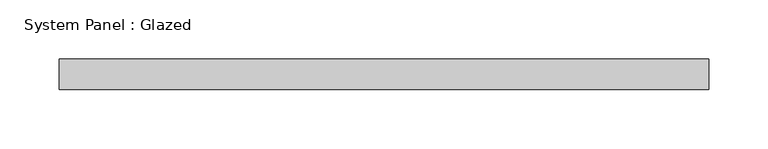
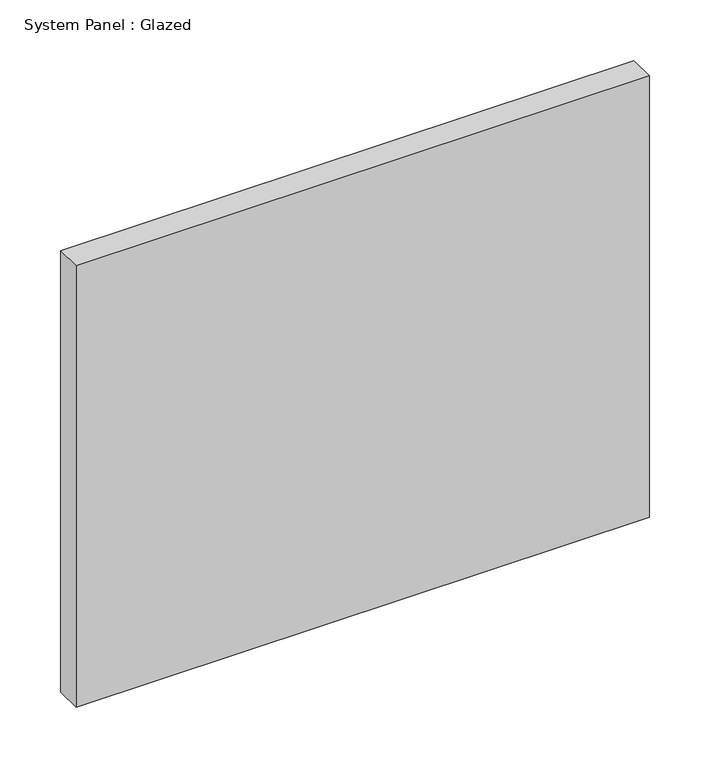
"""IFC4 building model written with IfcOpenShell, lengths in millimetres: plate geometry, System Panel : Glazed."""

from ifc_helpers import new_model, si_unit, origin, origin_with_axes, place, context, project, spatial, polyline, outline, extrude, source, transform, mapped, element, save


def system_panel_glazed_47dd2052(model_context):
    return source(origin(), model_context, "Body", "SweptSolid", [
        extrude(outline(polyline([(273.05, 19.05), (-273.05, 19.05), (-273.05, 44.45), (273.05, 44.45), (273.05, 19.05)])), origin_with_axes(), (0.0, 0.0, 1.0), 444.5),
    ])


if __name__ == "__main__":
    model = new_model("IFC4")
    model_context = context("Model", 3, world=origin())
    ifc_project = project(units=[si_unit("LENGTHUNIT", "METRE", prefix="MILLI")], contexts=[model_context])
    site = spatial("IfcSite", under=ifc_project)
    building = spatial("IfcBuilding", under=site)
    placement = place(None, origin())
    system_panel_glazed_shape = system_panel_glazed_47dd2052(model_context)
    element("IfcPlate", 1, ObjectType="System Panel : Glazed", at=placement, inside=building, context=model_context, shape_type="MappedRepresentation", body=[
        mapped(system_panel_glazed_shape, transform((0.0, 0.0, 0.0), x_axis=(1.0, 0.0, 0.0), y_axis=(0.0, 1.0, 0.0), z_axis=(0.0, 0.0, 1.0))),
    ])
    save(model, "model.ifc")

# Revit data of these elements
# Type "System Panel : Glazed"
#   Construction Type Id = "GSP4R"
#   Analytic Construction = "1/8 in Pilkington single glazing"
#   Visual Light Transmittance = 0.9
#   Solar Heat Gain Coefficient = 0.86
#   Heat Transfer Coefficient (U) = 1.18115 BTU/(h·ft²·°F)
#   Define Thermal Properties by = 1
# Element 1 (IfcPlate, "System Panel : Glazed")
#   Materials on its faces: "Glass"
# Materials
#   "Glass": class "Glass", colour RGB 0 128 192, transparency 0.75, Description = "Soda Lime Glass", Cost = 0
